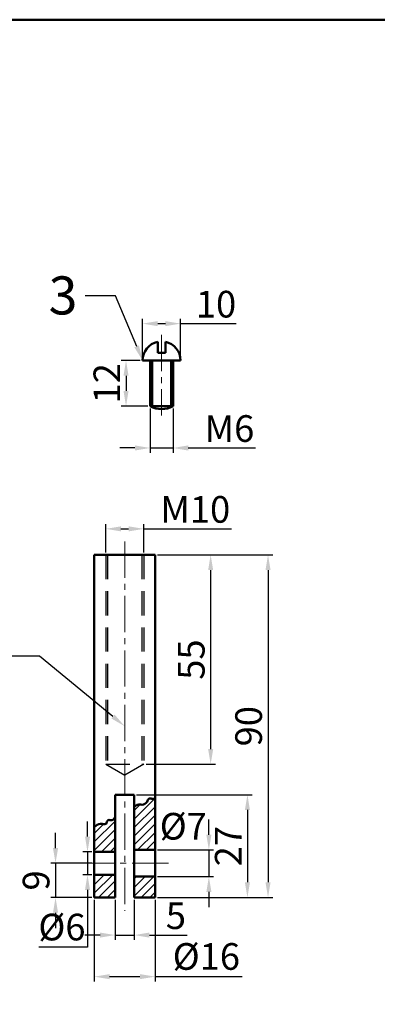
# Model space of a CAD drawing. Units: millimetres. Extents: x 376 to 1043, y -28 to 427.
# Tile 3 of 5: x 557 to 651, y 168 to 427. Entities that reach past the tile are written whole.
import ezdxf
from ezdxf import colors
from ezdxf.entities.mleader import LeaderData, LeaderLine
from ezdxf.math import Vec2, Vec3

# ---------------------------------------------------------------- set-up
doc = ezdxf.new("R2010")
doc.units = ezdxf.units.MM
doc.header["$LTSCALE"] = 0.5
doc.linetypes.add('CENTER2', pattern=[28.575, 19.05, -3.175, 3.175, -3.175])
doc.linetypes.add('DASHED', pattern=[19.05, 12.7, -6.35])
for name, color, linetype, lineweight in [('M-CNTR', 1, 'CENTER2', 18), ('M-DIMS', 2, 'Continuous', 25), ('M-HATC', 8, 'Continuous', 18), ('M-HIDN', 4, 'DASHED', 25), ('M-OUTL', 7, 'Continuous', 50)]:
    doc.layers.add(name, color=color, linetype=linetype, lineweight=lineweight)
doc.styles.get("Standard").update_dxf_attribs({"font": 'arial.ttf'})
doc.dimstyles.new('ISO-25', dxfattribs={"dimtxt": 7, "dimasz": 4, "dimexe": 1.25, "dimexo": 0.625, "dimtad": 1, "dimtoh": 1, "dimtxsty": 'Standard', "dimcen": 2.5, "dimadec": 0, "dimazin": 0, "dimtfac": 1, "dimtmove": 0, "dimatfit": 3, "dimfxl": 1, "dimarcsym": 0})

# ---------------------------------------------------------------- blocks, each defined once
blk = doc.blocks.new('*D1')
at = {"layer": 'Defpoints', "color": 0, "transparency": 16777216}
for p in [(599.64, 347.16), (589.64, 337.49), (599.64, 337.49)]:
    blk.add_point(p, dxfattribs=at)
at = {"layer": 'M-DIMS', "color": 0, "lineweight": -2, "transparency": 16777216}
for p, q in [((589.64, 338.12), (589.64, 348.41)), ((593.64, 347.16), (595.64, 347.16)), ((599.64, 338.12), (599.64, 348.41)), ((599.64, 347.16), (614.23, 347.16))]:
    blk.add_line(p, q, dxfattribs=at)
at = {"layer": 'M-DIMS', "color": 0, "transparency": 16777216}
for points in [[(593.64, 347.82), (593.64, 346.49), (589.64, 347.16)], [(595.64, 347.82), (595.64, 346.49), (599.64, 347.16)]]:
    blk.add_solid(points, dxfattribs=at)
at = {"layer": 'M-DIMS', "color": 0, "transparency": 16777216, "insert": (608.94, 351.36), "char_height": 7, "attachment_point": 5}
blk.add_mtext('10', dxfattribs=at)
blk = doc.blocks.new('*D2')
at = {"layer": 'Defpoints', "color": 0, "transparency": 16777216}
for p in [(589.64, 337.49), (585.29, 325.49), (591.64, 325.49)]:
    blk.add_point(p, dxfattribs=at)
at = {"layer": 'M-DIMS', "color": 0, "lineweight": -2, "transparency": 16777216}
for p, q in [((589.01, 337.49), (584.04, 337.49)), ((585.29, 333.49), (585.29, 329.49)), ((591.01, 325.49), (584.04, 325.49))]:
    blk.add_line(p, q, dxfattribs=at)
at = {"layer": 'M-DIMS', "color": 0, "transparency": 16777216}
for points in [[(584.63, 333.49), (585.96, 333.49), (585.29, 337.49)], [(584.63, 329.49), (585.96, 329.49), (585.29, 325.49)]]:
    blk.add_solid(points, dxfattribs=at)
at = {"layer": 'M-DIMS', "color": 0, "transparency": 16777216, "insert": (581.16, 331.49), "char_height": 7, "attachment_point": 5, "rotation": 90}
blk.add_mtext('12', dxfattribs=at)
blk = doc.blocks.new('*D3')
at = {"layer": 'Defpoints', "color": 0, "transparency": 16777216}
for p in [(591.64, 325.49), (597.64, 325.49), (597.64, 314.5)]:
    blk.add_point(p, dxfattribs=at)
at = {"layer": 'M-DIMS', "color": 0, "lineweight": -2, "transparency": 16777216}
for p, q in [((591.64, 324.87), (591.64, 313.25)), ((597.64, 324.87), (597.64, 313.25)), ((587.64, 314.5), (583.64, 314.5)), ((591.64, 314.5), (597.64, 314.5)), ((601.64, 314.5), (619.3, 314.5))]:
    blk.add_line(p, q, dxfattribs=at)
at = {"layer": 'M-DIMS', "color": 0, "transparency": 16777216}
for points in [[(587.64, 315.17), (587.64, 313.83), (591.64, 314.5)], [(601.64, 315.17), (601.64, 313.83), (597.64, 314.5)]]:
    blk.add_solid(points, dxfattribs=at)
at = {"layer": 'M-DIMS', "color": 0, "transparency": 16777216, "insert": (612.47, 318.7), "char_height": 7, "attachment_point": 5}
blk.add_mtext('M6', dxfattribs=at)
blk = doc.blocks.new('*U24')
at = {"layer": 'M-CNTR', "color": 0, "transparency": 16777216}
blk.add_line((0, 48.5), (0, -48.5), dxfattribs=at)
blk = doc.blocks.new('*U25')
at = {"layer": 'M-CNTR', "color": 0, "transparency": 16777216}
blk.add_line((6.25, 0), (-16.57, 0), dxfattribs=at)
blk = doc.blocks.new('*D27')
at = {"layer": 'Defpoints', "color": 0, "ltscale": 0.5, "transparency": 16777216}
for p in [(589.96, 293.26), (579.96, 286.42), (589.96, 286.42)]:
    blk.add_point(p, dxfattribs=at)
at = {"layer": 'M-DIMS', "color": 0, "lineweight": -2, "ltscale": 0.5, "transparency": 16777216}
for p, q in [((579.96, 287.04), (579.96, 294.51)), ((583.96, 293.26), (585.96, 293.26)), ((589.96, 287.04), (589.96, 294.51)), ((589.96, 293.26), (613.04, 293.26))]:
    blk.add_line(p, q, dxfattribs=at)
at = {"layer": 'M-DIMS', "color": 0, "ltscale": 0.5, "transparency": 16777216}
for points in [[(583.96, 293.92), (583.96, 292.59), (579.96, 293.26)], [(585.96, 293.92), (585.96, 292.59), (589.96, 293.26)]]:
    blk.add_solid(points, dxfattribs=at)
at = {"layer": 'M-DIMS', "color": 0, "ltscale": 0.5, "transparency": 16777216, "insert": (603.5, 297.46), "char_height": 7, "attachment_point": 5}
blk.add_mtext('M10', dxfattribs=at)
blk = doc.blocks.new('*D28')
at = {"layer": 'Defpoints', "color": 0, "ltscale": 0.5, "transparency": 16777216}
for p in [(592.96, 286.42), (589.96, 231.42), (607.53, 231.42)]:
    blk.add_point(p, dxfattribs=at)
at = {"layer": 'M-DIMS', "color": 0, "lineweight": -2, "ltscale": 0.5, "transparency": 16777216}
for p, q in [((593.58, 286.42), (608.78, 286.42)), ((607.53, 282.42), (607.53, 235.42)), ((590.58, 231.42), (608.78, 231.42))]:
    blk.add_line(p, q, dxfattribs=at)
at = {"layer": 'M-DIMS', "color": 0, "ltscale": 0.5, "transparency": 16777216}
for points in [[(606.87, 282.42), (608.2, 282.42), (607.53, 286.42)], [(606.87, 235.42), (608.2, 235.42), (607.53, 231.42)]]:
    blk.add_solid(points, dxfattribs=at)
at = {"layer": 'M-DIMS', "color": 0, "ltscale": 0.5, "transparency": 16777216, "insert": (603.35, 258.92), "char_height": 7, "attachment_point": 5, "rotation": 90}
blk.add_mtext('55', dxfattribs=at)
blk = doc.blocks.new('*D29')
at = {"layer": 'Defpoints', "color": 0, "ltscale": 0.5, "transparency": 16777216}
for p in [(601.18, 286.42), (592.96, 196.42), (622.61, 196.42)]:
    blk.add_point(p, dxfattribs=at)
at = {"layer": 'M-DIMS', "color": 0, "lineweight": -2, "ltscale": 0.5, "transparency": 16777216}
for p, q in [((601.81, 286.42), (623.86, 286.42)), ((622.61, 282.42), (622.61, 200.42)), ((593.58, 196.42), (623.86, 196.42))]:
    blk.add_line(p, q, dxfattribs=at)
at = {"layer": 'M-DIMS', "color": 0, "ltscale": 0.5, "transparency": 16777216}
for points in [[(621.94, 282.42), (623.28, 282.42), (622.61, 286.42)], [(621.94, 200.42), (623.28, 200.42), (622.61, 196.42)]]:
    blk.add_solid(points, dxfattribs=at)
at = {"layer": 'M-DIMS', "color": 0, "ltscale": 0.5, "transparency": 16777216, "insert": (618.41, 241.42), "char_height": 7, "attachment_point": 5, "rotation": 90}
blk.add_mtext('90', dxfattribs=at)
blk = doc.blocks.new('*D30')
at = {"layer": 'Defpoints', "color": 0, "ltscale": 0.5, "transparency": 16777216}
for p in [(587.46, 223.42), (597.41, 196.42), (617.2, 196.42)]:
    blk.add_point(p, dxfattribs=at)
at = {"layer": 'M-DIMS', "color": 0, "lineweight": -2, "ltscale": 0.5, "transparency": 16777216}
for p, q in [((588.08, 223.42), (618.45, 223.42)), ((617.2, 219.42), (617.2, 200.42)), ((598.03, 196.42), (618.45, 196.42))]:
    blk.add_line(p, q, dxfattribs=at)
at = {"layer": 'M-DIMS', "color": 0, "ltscale": 0.5, "transparency": 16777216}
for points in [[(616.53, 219.42), (617.86, 219.42), (617.2, 223.42)], [(616.53, 200.42), (617.86, 200.42), (617.2, 196.42)]]:
    blk.add_solid(points, dxfattribs=at)
at = {"layer": 'M-DIMS', "color": 0, "ltscale": 0.5, "transparency": 16777216, "insert": (613.06, 209.92), "char_height": 7, "attachment_point": 5, "rotation": 90}
blk.add_mtext('27', dxfattribs=at)
blk = doc.blocks.new('*D31')
at = {"layer": 'Defpoints', "color": 0, "ltscale": 0.5, "transparency": 16777216}
for p in [(576.96, 205.42), (566.77, 196.42), (576.96, 196.42)]:
    blk.add_point(p, dxfattribs=at)
at = {"layer": 'M-DIMS', "color": 0, "lineweight": -2, "ltscale": 0.5, "transparency": 16777216}
for p, q in [((566.77, 209.42), (566.77, 213.42)), ((576.33, 205.42), (565.52, 205.42)), ((566.77, 205.42), (566.77, 196.42)), ((576.33, 196.42), (565.52, 196.42)), ((566.77, 192.42), (566.77, 188.42))]:
    blk.add_line(p, q, dxfattribs=at)
at = {"layer": 'M-DIMS', "color": 0, "ltscale": 0.5, "transparency": 16777216}
for points in [[(566.1, 209.42), (567.44, 209.42), (566.77, 205.42)], [(566.1, 192.42), (567.44, 192.42), (566.77, 196.42)]]:
    blk.add_solid(points, dxfattribs=at)
at = {"layer": 'M-DIMS', "color": 0, "ltscale": 0.5, "transparency": 16777216, "insert": (562.57, 200.92), "char_height": 7, "attachment_point": 5, "rotation": 90}
blk.add_mtext('9', dxfattribs=at)
blk = doc.blocks.new('*D32')
at = {"layer": 'Defpoints', "color": 0, "ltscale": 0.5, "transparency": 16777216}
for p in [(576.96, 208.42), (575.17, 202.42), (576.96, 202.42)]:
    blk.add_point(p, dxfattribs=at)
at = {"layer": 'M-DIMS', "color": 0, "lineweight": -2, "ltscale": 0.5, "transparency": 16777216}
for p, q in [((575.17, 212.42), (575.17, 216.42)), ((576.33, 208.42), (573.92, 208.42)), ((575.17, 208.42), (575.17, 202.42)), ((576.33, 202.42), (573.92, 202.42)), ((575.17, 198.42), (575.17, 183.36)), ((575.17, 183.36), (562.35, 183.36))]:
    blk.add_line(p, q, dxfattribs=at)
at = {"layer": 'M-DIMS', "color": 0, "ltscale": 0.5, "transparency": 16777216}
for points in [[(574.51, 212.42), (575.84, 212.42), (575.17, 208.42)], [(574.51, 198.42), (575.84, 198.42), (575.17, 202.42)]]:
    blk.add_solid(points, dxfattribs=at)
at = {"layer": 'M-DIMS', "color": 0, "ltscale": 0.5, "transparency": 16777216, "insert": (568.45, 187.76), "char_height": 7, "attachment_point": 5}
blk.add_mtext('%%C6', dxfattribs=at)
blk = doc.blocks.new('*D33')
at = {"layer": 'Defpoints', "color": 0, "ltscale": 0.5, "transparency": 16777216}
for p in [(592.96, 208.92), (592.96, 201.92), (607.07, 201.92)]:
    blk.add_point(p, dxfattribs=at)
at = {"layer": 'M-DIMS', "color": 0, "lineweight": -2, "ltscale": 0.5, "transparency": 16777216}
for p, q in [((607.07, 212.92), (607.07, 216.92)), ((593.58, 208.92), (608.32, 208.92)), ((607.07, 208.92), (607.07, 201.92)), ((593.58, 201.92), (608.32, 201.92)), ((607.07, 197.92), (607.07, 193.92))]:
    blk.add_line(p, q, dxfattribs=at)
at = {"layer": 'M-DIMS', "color": 0, "ltscale": 0.5, "transparency": 16777216}
for points in [[(606.4, 212.92), (607.74, 212.92), (607.07, 208.92)], [(606.4, 197.92), (607.74, 197.92), (607.07, 201.92)]]:
    blk.add_solid(points, dxfattribs=at)
at = {"layer": 'M-DIMS', "color": 0, "ltscale": 0.5, "transparency": 16777216, "insert": (600.34, 214.24), "char_height": 7, "attachment_point": 5}
blk.add_mtext('%%C7', dxfattribs=at)
blk = doc.blocks.new('*D34')
at = {"layer": 'Defpoints', "color": 0, "ltscale": 0.5, "transparency": 16777216}
for p in [(582.46, 196.42), (587.46, 196.42), (587.46, 186.56)]:
    blk.add_point(p, dxfattribs=at)
at = {"layer": 'M-DIMS', "color": 0, "lineweight": -2, "ltscale": 0.5, "transparency": 16777216}
for p, q in [((582.46, 195.79), (582.46, 185.31)), ((587.46, 195.79), (587.46, 185.31)), ((578.46, 186.56), (574.46, 186.56)), ((582.46, 186.56), (587.46, 186.56)), ((591.46, 186.56), (601.35, 186.56))]:
    blk.add_line(p, q, dxfattribs=at)
at = {"layer": 'M-DIMS', "color": 0, "ltscale": 0.5, "transparency": 16777216}
for points in [[(578.46, 187.23), (578.46, 185.9), (582.46, 186.56)], [(591.46, 187.23), (591.46, 185.9), (587.46, 186.56)]]:
    blk.add_solid(points, dxfattribs=at)
at = {"layer": 'M-DIMS', "color": 0, "ltscale": 0.5, "transparency": 16777216, "insert": (598.4, 190.75), "char_height": 7, "attachment_point": 5}
blk.add_mtext('5', dxfattribs=at)
blk = doc.blocks.new('*D35')
at = {"layer": 'Defpoints', "color": 0, "ltscale": 0.5, "transparency": 16777216}
for p in [(576.96, 196.42), (592.96, 196.42), (592.96, 175.65)]:
    blk.add_point(p, dxfattribs=at)
at = {"layer": 'M-DIMS', "color": 0, "lineweight": -2, "ltscale": 0.5, "transparency": 16777216}
for p, q in [((576.96, 195.79), (576.96, 174.4)), ((592.96, 195.79), (592.96, 174.4)), ((580.96, 175.65), (588.96, 175.65)), ((592.96, 175.65), (615.85, 175.65))]:
    blk.add_line(p, q, dxfattribs=at)
at = {"layer": 'M-DIMS', "color": 0, "ltscale": 0.5, "transparency": 16777216}
for points in [[(580.96, 176.31), (580.96, 174.98), (576.96, 175.65)], [(588.96, 176.31), (588.96, 174.98), (592.96, 175.65)]]:
    blk.add_solid(points, dxfattribs=at)
at = {"layer": 'M-DIMS', "color": 0, "ltscale": 0.5, "transparency": 16777216, "insert": (606.4, 180.04), "char_height": 7, "attachment_point": 5}
blk.add_mtext('%%C16', dxfattribs=at)

msp = doc.modelspace()

# ---------------------------------------------------------------- hatches: boundary and pattern name
at = {"layer": 'M-HATC', "ltscale": 0.5}
h = msp.add_hatch(dxfattribs=at)
h.set_pattern_fill('ANSI31', color=256, scale=0.5)
edge = h.paths.add_edge_path()
edge.add_spline(control_points=[(582.458, 217.652), (582.207, 217.218), (581.773, 216.465), (580.351, 217.071), (580.197, 215.285), (578.284, 216.184), (577.435, 215.344), (576.958, 214.872)], knot_values=[0, 0, 0, 0, 1.3025469, 2.260803, 3.3332508, 4.7909835, 6.6629684, 6.6629684, 6.6629684, 6.6629684], degree=3, periodic=0)
edge.add_line((576.958, 214.872), (576.958, 208.419))
edge.add_line((576.958, 208.419), (582.458, 208.419))
edge.add_line((582.458, 208.419), (582.458, 217.652))
edge = h.paths.add_edge_path()
edge.add_spline(control_points=[(592.958, 222.386), (592.675, 222.368), (592.146, 222.333), (591.142, 222.577), (590.893, 221.247), (589.667, 220.669), (588.375, 220.976), (587.768, 220.5), (587.458, 220.256)], knot_values=[0, 0, 0, 0, 0.8821612, 1.6498541, 2.5550205, 4.1264864, 5.1929388, 6.3132072, 6.3132072, 6.3132072, 6.3132072], degree=3, periodic=0)
edge.add_line((587.458, 220.256), (587.458, 208.919))
edge.add_line((587.458, 208.919), (592.958, 208.919))
edge.add_line((592.958, 208.919), (592.958, 222.386))
h.paths.add_polyline_path([(582.458, 202.419), (576.958, 202.419), (576.958, 196.419), (582.458, 196.419)])
h.paths.add_polyline_path([(592.958, 201.919), (587.458, 201.919), (587.458, 196.419), (592.958, 196.419)])

# ---------------------------------------------------------------- linework, layer by layer
at = {"layer": 'M-CNTR'}
msp.add_line((594.639, 344.224), (594.639, 323.022), dxfattribs=at)
at = {"layer": 'M-HIDN'}
for p, q in [((579.958, 286.419), (579.958, 231.419)), ((580.458, 286.419), (580.458, 231.419)), ((589.458, 286.419), (589.458, 231.419)), ((589.958, 286.419), (589.958, 231.419)), ((579.958, 231.419), (589.958, 231.419)), ((579.958, 231.419), (584.958, 228.532)), ((589.958, 231.419), (584.958, 228.532))]:
    msp.add_line(p, q, dxfattribs=at)
at = {"layer": 'M-OUTL'}
for p, q in [((593.639, 339.492), (593.639, 342.391)), ((595.639, 339.492), (595.639, 342.391)), ((594.639, 339.492), (593.639, 339.492)), ((594.639, 339.492), (595.639, 339.492)), ((589.639, 337.492), (599.639, 337.492)), ((591.639, 325.492), (591.639, 337.492)), ((592.139, 325.492), (592.139, 337.492)), ((597.139, 337.492), (597.139, 325.492)), ((597.639, 337.492), (597.639, 325.492)), ((597.639, 325.492), (591.639, 325.492)), ((576.958, 286.419), (592.958, 286.419)), ((576.958, 196.419), (576.958, 286.419)), ((592.958, 286.419), (592.958, 196.419)), ((582.458, 208.419), (576.958, 208.419)), ((592.958, 208.919), (587.458, 208.919)), ((582.458, 202.419), (576.958, 202.419)), ((592.958, 201.919), (587.458, 201.919)), ((582.458, 196.419), (576.958, 196.419)), ((592.958, 196.419), (587.458, 196.419))]:
    msp.add_line(p, q, dxfattribs=at)
at = {"layer": 'M-OUTL', "ltscale": 0.5}
for p, q in [((587.458, 223.419), (582.458, 223.419)), ((582.458, 223.419), (582.458, 196.419)), ((587.458, 196.419), (587.458, 223.419))]:
    msp.add_line(p, q, dxfattribs=at)
msp.add_lwpolyline([(376.448, 426.986), (1042.916, 426.986), (1042.916, -28.377), (376.448, -28.377)], close=True, dxfattribs=at)
at = {"layer": 'M-OUTL'}
for centre, radius, start, end in [((594.639, 337.492), 5, 101.53696, 180), ((594.639, 337.492), 5, 0, 78.46304), ((594.639, 330.688), 6, 240, 300)]:
    msp.add_arc(centre, radius, start, end, dxfattribs=at)
at = {"layer": 'M-OUTL', "ltscale": 0.5}
for points, knots in [([(587.458, 220.256), (587.768, 220.5), (588.375, 220.976), (589.667, 220.669), (590.893, 221.247), (591.142, 222.577), (592.146, 222.333), (592.675, 222.368), (592.958, 222.386)], [0, 0, 0, 0, 1.1202684, 2.1867208, 3.7581867, 4.6633531, 5.431046, 6.3132072, 6.3132072, 6.3132072, 6.3132072]), ([(576.958, 214.872), (577.435, 215.344), (578.284, 216.184), (580.197, 215.285), (580.351, 217.071), (581.773, 216.465), (582.207, 217.218), (582.458, 217.652)], [0, 0, 0, 0, 1.8719849, 3.3297176, 4.4021655, 5.3604215, 6.6629684, 6.6629684, 6.6629684, 6.6629684])]:
    msp.add_open_spline(points, degree=3, knots=knots, dxfattribs=at)

# ---------------------------------------------------------------- block references
at = {"layer": 'M-CNTR'}
for name, p in [('*U24', (584.958, 241.419)), ('*U25', (590.208, 205.419))]:
    msp.add_blockref(name, p, dxfattribs=at)

# ---------------------------------------------------------------- dimensions: what is measured, and where the dimension line sits
at = {"layer": 'M-DIMS'}
dim = msp.add_linear_dim(base=(599.639, 347.156), p1=(589.639, 337.492), p2=(599.639, 337.492), dimstyle='ISO-25', override={"dimclrd": 0, "dimclre": 0, "dimclrt": 0}, dxfattribs=at)
dim.commit()
dim.dimension.update_dxf_attribs({"geometry": '*D1', "text_midpoint": (608.936, 351.355)})
dim = msp.add_linear_dim(base=(585.295, 325.492), p1=(589.639, 337.492), p2=(591.639, 325.492), angle=90, dimstyle='ISO-25', override={"dimclrd": 0, "dimclre": 0, "dimclrt": 0}, dxfattribs=at)
dim.commit()
dim.dimension.update_dxf_attribs({"geometry": '*D2', "text_midpoint": (581.155, 331.492)})
dim = msp.add_linear_dim(base=(597.639, 314.501), p1=(591.639, 325.492), p2=(597.639, 325.492), text='M<>', dimstyle='ISO-25', override={"dimclrd": 0, "dimclre": 0, "dimclrt": 0}, dxfattribs=at)
dim.commit()
dim.dimension.update_dxf_attribs({"geometry": '*D3', "text_midpoint": (612.469, 318.7)})
at = {"layer": 'M-DIMS', "ltscale": 0.5}
for base, p1, p2, text, picture, middle in [((589.958, 293.258), (579.958, 286.419), (589.958, 286.419), 'M<>', '*D27', (603.497, 297.457)), ((592.958, 175.645), (576.958, 196.419), (592.958, 196.419), '%%C<>', '*D35', (606.402, 180.04))]:
    dim = msp.add_linear_dim(base=base, p1=p1, p2=p2, text=text, dimstyle='ISO-25', override={"dimclrd": 0, "dimclre": 0, "dimclrt": 0}, dxfattribs=at)
    dim.commit()
    dim.dimension.update_dxf_attribs({"geometry": picture, "text_midpoint": middle})
for base, p1, p2, picture, middle in [((607.532, 231.419), (592.958, 286.419), (589.958, 231.419), '*D28', (603.348, 258.919)), ((622.609, 196.419), (601.183, 286.419), (592.958, 196.419), '*D29', (618.41, 241.419))]:
    dim = msp.add_linear_dim(base=base, p1=p1, p2=p2, angle=90, dimstyle='ISO-25', override={"dimclrd": 0, "dimclre": 0, "dimclrt": 0}, dxfattribs=at)
    dim.commit()
    dim.dimension.update_dxf_attribs({"geometry": picture, "text_midpoint": middle})
for base, p1, p2, picture, middle in [((617.197, 196.419), (587.458, 223.419), (597.409, 196.419), '*D30', (617.197, 209.919)), ((566.769, 196.419), (576.958, 205.419), (576.958, 196.419), '*D31', (566.769, 200.919))]:
    dim = msp.add_linear_dim(base=base, p1=p1, p2=p2, angle=90, dimstyle='ISO-25', override={"dimclrd": 0, "dimclre": 0, "dimclrt": 0}, dxfattribs=at)
    dim.commit()
    dim.dimension.update_dxf_attribs({"geometry": picture, "text_midpoint": middle, "dimtype": 160})
for base, p1, p2, override, picture, middle in [((607.071, 201.919), (592.958, 208.919), (592.958, 201.919), {"dimclrd": 0, "dimclre": 0, "dimclrt": 0, "dimtmove": 2}, '*D33', (600.344, 214.238)), ((575.173, 202.419), (576.958, 208.419), (576.958, 202.419), {"dimclrd": 0, "dimclre": 0, "dimclrt": 0}, '*D32', (568.448, 183.364))]:
    dim = msp.add_linear_dim(base=base, p1=p1, p2=p2, angle=90, text='%%C<>', dimstyle='ISO-25', override=override, dxfattribs=at)
    dim.commit()
    dim.dimension.update_dxf_attribs({"geometry": picture, "text_midpoint": middle, "dimtype": 160})
dim = msp.add_linear_dim(base=(587.458, 186.564), p1=(582.458, 196.419), p2=(587.458, 196.419), dimstyle='ISO-25', override={"dimclrd": 0, "dimclre": 0, "dimclrt": 0}, dxfattribs=at)
dim.commit()
dim.dimension.update_dxf_attribs({"geometry": '*D34', "text_midpoint": (598.403, 190.749)})

# ---------------------------------------------------------------- leaders
at = {"layer": 'M-DIMS'}
ml = msp.add_multileader_mtext('Standard', dxfattribs=at)
ml.set_content('3', color=256)
ml.set_leader_properties()
ml.build(insert=Vec2(0, 0))
ctx = ml.context
ctx.base_point, ctx.char_height, ctx.plane_origin = Vec3(563.981, 354.473), 10, Vec3(589.639, 337.492)
ctx.text_align_type = 2
notes = []
notes.append((ctx, [(0, (1, 1, 0), (582.529, 354.473), (-1, 0), 8, [(0, [(589.639, 337.492)], 0, [])])]))
ctx.mtext.insert, ctx.mtext.alignment, ctx.mtext.flow_direction = Vec3(572.529, 359.562), 3, 5
at = {"layer": 'M-DIMS', "ltscale": 0.5}
ml = msp.add_multileader_mtext('Standard', dxfattribs=at)
ml.set_content('13', color=256)
ml.set_leader_properties()
ml.build(insert=Vec2(0, 0))
ctx = ml.context
ctx.base_point, ctx.char_height, ctx.plane_origin = Vec3(537.2, 259.791), 10, Vec3(584.958, 241.419)
ctx.text_align_type = 2
notes.append((ctx, [(0, (1, 1, 0), (562.584, 259.791), (-1, 0), 8, [(0, [(584.958, 241.419)], 0, [])])]))
ctx.mtext.insert, ctx.mtext.alignment, ctx.mtext.flow_direction = Vec3(552.584, 264.879), 3, 5
for ctx, leaders in notes:
    for number, flags, end, landing, length, lines in leaders:
        leader = LeaderData()
        leader.index, (leader.has_last_leader_line, leader.has_dogleg_vector, leader.attachment_direction) = number, flags
        leader.last_leader_point, leader.dogleg_vector, leader.dogleg_length = Vec3(end), Vec3(landing), length
        for number, points, colour, breaks in lines:
            line = LeaderLine()
            line.index, line.vertices, line.color, line.breaks = number, Vec3.list(points), colors.encode_raw_color(colour), breaks
            leader.lines.append(line)
        ctx.leaders.append(leader)

doc.saveas('drawing.dxf')
